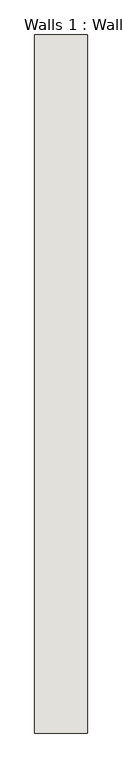
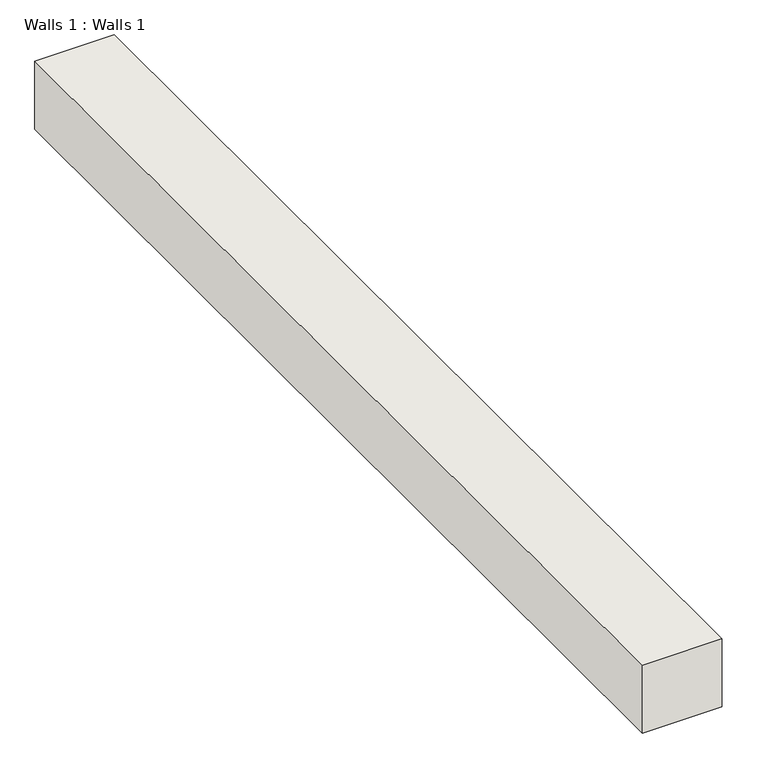
"""IFC4 building model written with IfcOpenShell, lengths in millimetres: wall geometry, Walls 1 : Walls 1."""

from ifc_helpers import new_model, si_unit, frame, origin, place, context, project, spatial, polyline, outline, extrude, source, transform, mapped, element, save


def walls_1_walls_1_bd393664(model_context):
    return source(origin(), model_context, "Body", "SweptSolid", [
        extrude(outline(polyline([(-3125.3625081, -8837.7409243), (-3125.3625081, -798.6874979), (-2519.5479903, -798.6874979), (-2519.5479903, -8837.7409243), (-3125.3625081, -8837.7409243)])), frame((0.0, 0.0, 5548.8403036), z_axis=(0.0, 0.0, 1.0), x_axis=(1.0, 0.0, 0.0)), (0.0, 0.0, 1.0), 548.3596964),
    ])


if __name__ == "__main__":
    model = new_model("IFC4")
    model_context = context("Model", 3, world=origin())
    ifc_project = project(units=[si_unit("LENGTHUNIT", "METRE", prefix="MILLI")], contexts=[model_context])
    site = spatial("IfcSite", under=ifc_project)
    building = spatial("IfcBuilding", under=site)
    placement = place(None, origin())
    walls_1_walls_1_shape = walls_1_walls_1_bd393664(model_context)
    element("IfcWall", 1, ObjectType="Walls 1 : Walls 1", at=placement, inside=building, context=model_context, shape_type="MappedRepresentation", body=[
        mapped(walls_1_walls_1_shape, transform((0.0, 0.0, 0.0), x_axis=(1.0, 0.0, 0.0), y_axis=(0.0, 1.0, 0.0), z_axis=(0.0, 0.0, 1.0))),
    ])
    save(model, "model.ifc")

# Revit data of these elements
# Element 1 (IfcWall, "Walls 1 : Walls 1")
#   Materials on its faces: "Default Wall"
# Materials
#   "Default Wall": colour RGB 80 80 80, transparency 0
